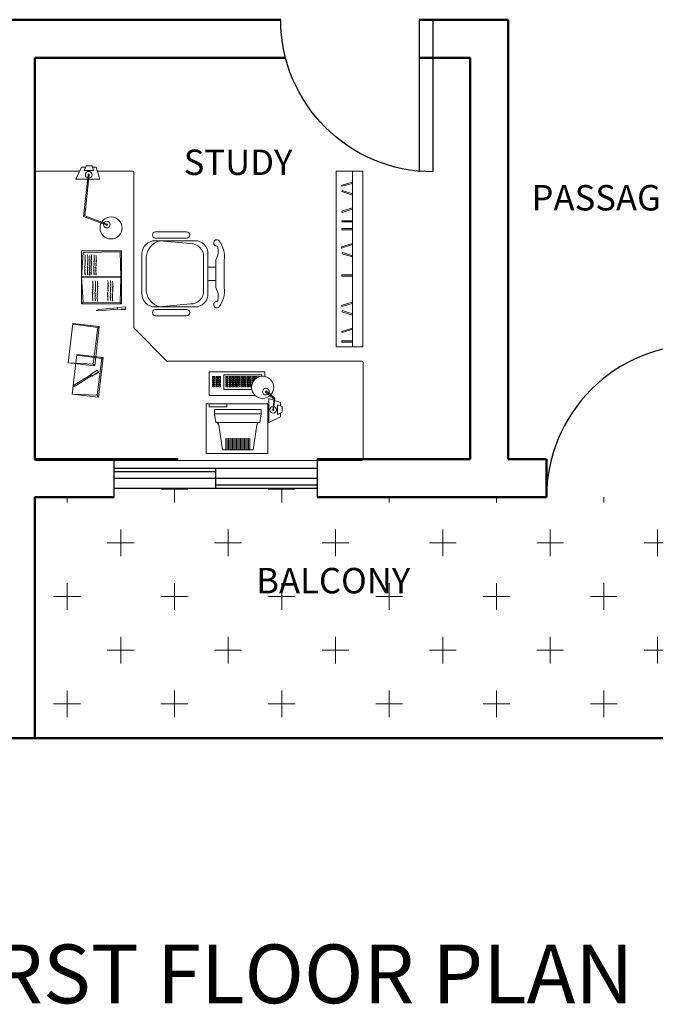
# Model space of a CAD drawing. Units: millimetres. Extents: x -857 to 54106, y -13666 to 13947.
# Tile 17 of 41: x 24780 to 28540, y 2329 to 8154. Entities that reach past the tile are written whole.
import ezdxf

# ---------------------------------------------------------------- set-up
doc = ezdxf.new("R2010")
doc.units = ezdxf.units.MM
for name, color, linetype, lineweight in [('A-ANNO-TEXT', 7, 'Continuous', 25), ('A-AREA-IDEN', 3, 'Continuous', 18), ('A-DOOR', 1, 'Continuous', 25), ('A-FLOR-PATT', 252, 'Continuous', 13), ('A-FURN', 21, 'Continuous', 18), ('A-GLAZ', 4, 'Continuous', 25), ('A-WALL', 7, 'Continuous', 50)]:
    doc.layers.add(name, color=color, linetype=linetype, lineweight=lineweight)
doc.styles.get("Standard").update_dxf_attribs({"font": 'arial.ttf'})

# ---------------------------------------------------------------- blocks, each defined once
blk = doc.blocks.new('DOOR-900')
blk.add_line((11417.3, 9811.5), (12317.3, 9811.5))
blk.add_arc((11417.3, 9811.5), 900, 0, 90)
blk = doc.blocks.new('WIN-1200')
for p, q in [((9371.3, 11750.2), (10571.3, 11750.2)), ((9371.3, 11731.7), (9971.3, 11731.7)), ((9971.3, 11750.2), (9971.3, 11630.7)), ((9371.3, 11691.7), (10571.3, 11691.7)), ((9971.3, 11651.7), (10571.3, 11651.7)), ((10571.3, 11630.7), (9371.3, 11630.7))]:
    blk.add_line(p, q)
for points in [[(9371.3, 11579.2), (9371.3, 11804.2)], [(10571.3, 11804.2), (10571.3, 11579.2)]]:
    blk.add_lwpolyline(points)

msp = doc.modelspace()

# ---------------------------------------------------------------- hatches: boundary and pattern name
at = {"layer": 'A-FLOR-PATT'}
h = msp.add_hatch(dxfattribs=at)
h.set_pattern_fill('CROSS', color=256, scale=50)
h.set_pattern_definition([(0, (11962.88, -2561.3), (317.5, 317.5), [158.75, -476.25]), (90, (12042.26, -2640.7), (-317.5, 317.5), [158.75, -476.25])])
h.paths.add_polyline_path([(29079.919, 5329.231), (28716.385, 5329.231), (27076.385, 5329.231), (26996.385, 5329.231), (26539.053, 5329.231), (26539.053, 5380.706), (25339.053, 5380.706), (25339.053, 5329.231), (24870.079, 5329.231), (24870.079, 3903.799), (29079.919, 3903.799)])

# ---------------------------------------------------------------- linework, layer by layer
at = {"layer": 'A-DOOR'}
msp.add_line((27143.761, 8154.231), (27143.761, 7254.231), dxfattribs=at)
at = {"layer": 'A-FURN'}
for p, q in [((25160.508, 7261.556), (25173.98, 7289.341)), ((25208.191, 7289.341), (25173.98, 7289.341)), ((25208.191, 7289.341), (25217.357, 7261.556)), ((25112.268, 7211.399), (25145.95, 7280.862)), ((25169.869, 7280.862), (25145.95, 7280.862)), ((25184.32, 7235.602), (25158.173, 6990.396)), ((25217.357, 7261.556), (25160.508, 7261.556)), ((25191.68, 7238.315), (25165.182, 6994.061)), ((25231.476, 7280.862), (25210.988, 7280.862)), ((25231.476, 7280.862), (25254.392, 7211.399)), ((26652.793, 7258.702), (26652.793, 6219.198)), ((26652.793, 7258.702), (26810.205, 7258.702)), ((26748.886, 7258.702), (26748.886, 6219.198)), ((26810.205, 6219.198), (26810.205, 7258.702)), ((25254.392, 7211.399), (25112.268, 7211.399)), ((25158.173, 6990.396), (25291.756, 6940.082)), ((25165.182, 6994.061), (25298.184, 6944.578)), ((25581.356, 6899.415), (25767.4, 6899.415)), ((25581.356, 6861.617), (25767.4, 6861.617)), ((25155.775, 6777.447), (25146.069, 6630.683)), ((25375.038, 6780.342), (25155.775, 6777.447)), ((25375.038, 6780.342), (25378.51, 6633.881)), ((25893.633, 6690.024), (25939.644, 6690.024)), ((25378.51, 6633.881), (25146.069, 6633.881)), ((25155.775, 6483.92), (25146.069, 6630.683)), ((25375.038, 6481.025), (25378.51, 6627.485)), ((25378.51, 6627.485), (25381.257, 6630.659)), ((25893.633, 6611.58), (25939.644, 6611.58)), ((25146.069, 6473.796), (25155.775, 6483.92)), ((25375.038, 6481.025), (25155.775, 6483.92)), ((25381.399, 6473.796), (25375.038, 6481.025)), ((25246.61, 6439.514), (25232.761, 6433.905)), ((25232.761, 6433.905), (25247.32, 6431.702)), ((25358.654, 6449.693), (25246.61, 6439.514)), ((25359.364, 6441.881), (25247.32, 6431.702)), ((25358.465, 6451.781), (25405.161, 6456.024)), ((25358.654, 6449.693), (25358.465, 6451.781)), ((25359.544, 6438.967), (25358.57, 6449.686)), ((25406.325, 6443.217), (25359.544, 6438.967)), ((25404.946, 6443.883), (25382.156, 6441.813)), ((25382.156, 6441.813), (25382.459, 6438.476)), ((25405.249, 6440.546), (25382.459, 6438.476)), ((25404.946, 6443.883), (25405.249, 6440.546)), ((25405.161, 6456.024), (25406.325, 6443.217)), ((25581.356, 6439.986), (25767.4, 6439.986)), ((25096.866, 6353.896), (25094.021, 6356.983)), ((25242.011, 6334.005), (25096.866, 6353.896)), ((25581.356, 6402.189), (25767.4, 6402.189)), ((25242.011, 6334.005), (25214.52, 6116.453)), ((25249.908, 6339.515), (25242.011, 6334.005)), ((25650.994, 6134.713), (25454.885, 6330.671)), ((26652.793, 6219.198), (26810.205, 6219.198)), ((25214.52, 6116.453), (25067.595, 6123.284)), ((25120.179, 6170.198), (25117.333, 6173.285)), ((25265.323, 6150.308), (25120.179, 6170.198)), ((25223.49, 6105.672), (25214.52, 6116.453)), ((25265.323, 6150.308), (25237.833, 5932.755)), ((25265.323, 6150.308), (25273.22, 6155.817)), ((25199.076, 6055.795), (25238.723, 6080.829)), ((25245.589, 6069.956), (25205.871, 6044.876)), ((25244.058, 6069.921), (25224.709, 6057.704)), ((25245.846, 6067.088), (25226.498, 6054.871)), ((25238.723, 6080.829), (25245.589, 6069.956)), ((25244.058, 6069.921), (25245.846, 6067.088)), ((26229.928, 6070.027), (25901.209, 6070.027)), ((25901.209, 6070.027), (25901.209, 5931.619)), ((26229.928, 6043.131), (26229.928, 6070.027)), ((25200.196, 6054.022), (25105.067, 5993.955)), ((25204.384, 6047.389), (25109.255, 5987.322)), ((25200.196, 6054.022), (25199.076, 6055.795)), ((25205.871, 6044.876), (25200.124, 6053.977)), ((25224.709, 6057.704), (25226.498, 6054.871)), ((26212.627, 6052.726), (25987.714, 6052.726)), ((25987.714, 6052.726), (25987.714, 5966.221)), ((26212.627, 6044.227), (26212.627, 6052.726)), ((25105.067, 5993.955), (25095.29, 5982.656)), ((25095.29, 5982.656), (25109.255, 5987.322)), ((25987.714, 5966.221), (26152.903, 5966.221)), ((26285.149, 5908.373), (26234.835, 5949.996)), ((26288.815, 5915.382), (26239.332, 5956.423)), ((25237.833, 5932.755), (25090.907, 5939.586)), ((25246.802, 5921.974), (25237.833, 5932.755)), ((25901.209, 5931.619), (26171.815, 5931.619)), ((26253.814, 5912.631), (26253.814, 5770.508)), ((26323.277, 5889.716), (26253.814, 5912.631)), ((26278.016, 5842.559), (26285.149, 5908.373)), ((26280.73, 5849.919), (26288.815, 5915.382)), ((26323.277, 5889.716), (26323.277, 5869.227)), ((26247.151, 5881.979), (25883.829, 5881.979)), ((25883.829, 5881.979), (25883.829, 5587.862)), ((25901.13, 5881.979), (25901.13, 5864.678)), ((25901.13, 5864.678), (26004.936, 5864.678)), ((26207.734, 5847.871), (25931.613, 5847.871)), ((25931.613, 5847.871), (25931.613, 5823.408)), ((26004.936, 5864.678), (26004.936, 5881.979)), ((26207.734, 5823.408), (26207.734, 5847.871)), ((26247.151, 5587.862), (26247.151, 5881.979)), ((26303.97, 5875.597), (26303.97, 5818.747)), ((26331.756, 5866.43), (26303.97, 5875.597)), ((26303.97, 5818.747), (26331.756, 5832.22)), ((26323.277, 5828.109), (26323.277, 5804.189)), ((26331.756, 5866.43), (26331.756, 5832.22)), ((25931.613, 5823.408), (26207.734, 5823.408)), ((25931.613, 5823.408), (25939.595, 5770.488)), ((26199.982, 5770.488), (25939.595, 5770.488)), ((26199.982, 5770.488), (26207.734, 5823.408)), ((26253.814, 5770.508), (26323.277, 5804.189)), ((25978.907, 5610.358), (25957.543, 5756.207)), ((26160.67, 5610.358), (26182.034, 5756.207)), ((25999.538, 5610.358), (25999.538, 5679.223)), ((26007.383, 5610.358), (26007.383, 5679.223)), ((26015.227, 5610.358), (26015.227, 5679.223)), ((26023.071, 5610.358), (26023.071, 5679.223)), ((26030.916, 5610.358), (26030.916, 5679.223)), ((26038.76, 5610.358), (26038.76, 5679.223)), ((26046.604, 5610.358), (26046.604, 5679.223)), ((26054.449, 5610.358), (26054.449, 5679.223)), ((26054.449, 5610.358), (26054.449, 5679.223)), ((26062.293, 5610.358), (26062.293, 5679.223)), ((26070.137, 5610.358), (26070.137, 5679.223)), ((26077.982, 5610.358), (26077.982, 5679.223)), ((26085.826, 5610.358), (26085.826, 5679.223)), ((26093.67, 5610.358), (26093.67, 5679.223)), ((26101.515, 5610.358), (26101.515, 5679.223)), ((26109.359, 5610.358), (26109.359, 5679.223)), ((26117.204, 5610.358), (26117.204, 5679.223)), ((26125.048, 5610.358), (26125.048, 5679.223)), ((26132.892, 5610.358), (26132.892, 5679.223)), ((26140.737, 5610.358), (26140.737, 5679.223)), ((25978.907, 5610.358), (26160.67, 5610.358)), ((25883.829, 5587.862), (26247.151, 5587.862))]:
    msp.add_line(p, q, dxfattribs=at)
for points in [[(25447.04, 5546.387), (24874.403, 5546.387, -0.41421356), (24866.558, 5554.231), (24866.558, 7250.857, -0.41421356), (24874.403, 7258.702), (25135.205, 7258.702)], [(25238.787, 7258.702), (25447.04, 7258.702, -0.41421356), (25454.885, 7250.857), (25454.885, 6330.671)], [(25502.985, 6650.802), (25502.985, 6768.467, -0.41421356), (25581.428, 6846.911), (25816.759, 6846.911, -0.41837619), (25893.633, 6768.467), (25893.633, 6650.802)], [(25527.65, 6650.802), (25527.65, 6750.867, -0.28027969), (25606.094, 6846.911), (25791.171, 6829.311, -0.41837619), (25868.045, 6750.867), (25868.045, 6650.802)], [(25956.196, 6850.36, -0.20706567), (25990.378, 6731.064), (25990.378, 6650.802)], [(25949.073, 6814.782, -0.21457838), (25939.644, 6731.387), (25939.644, 6650.802)], [(25502.985, 6650.802), (25502.985, 6533.137, 0.41421356), (25581.428, 6454.693), (25816.759, 6454.693, 0.41837619), (25893.633, 6533.137), (25893.633, 6650.802)], [(25527.65, 6650.802), (25527.65, 6550.736, 0.28027969), (25606.094, 6454.693), (25791.171, 6472.293, 0.41837619), (25868.045, 6550.736), (25868.045, 6650.802)], [(25949.073, 6486.822, 0.21457838), (25939.644, 6570.217), (25939.644, 6650.802)], [(25956.196, 6451.244, 0.20706567), (25990.378, 6570.54), (25990.378, 6650.802)], [(25650.994, 6134.713), (26804.658, 6134.713, -0.41421356), (26812.503, 6126.869), (26812.503, 5554.231, -0.41421356), (26804.658, 5546.387), (25447.04, 5546.387)]]:
    msp.add_lwpolyline(points, format="xyb", dxfattribs=at)
for points in [[(26748.886, 7185.97), (26686.412, 7169.063), (26685.22, 7175.896), (26748.886, 7193.127)], [(26748.886, 7116.919), (26686.222, 7136.927), (26687.616, 7143.722), (26748.886, 7124.159)], [(26748.886, 7040.642), (26686.222, 7020.633), (26687.616, 7013.838), (26748.886, 7033.401)], [(26748.886, 6958.009), (26685.22, 6958.009), (26685.22, 6964.946), (26748.886, 6964.946)], [(26748.886, 6911.186), (26685.22, 6911.186), (26685.22, 6918.122), (26748.886, 6918.122)], [(26748.886, 6830.798), (26682.756, 6809.683), (26684.15, 6802.888), (26748.886, 6823.558)], [(26748.886, 6750.443), (26687.955, 6769.898), (26689.349, 6776.693), (26748.886, 6757.683)], [(26748.886, 6637.18), (26685.22, 6637.18), (26685.22, 6644.116), (26748.886, 6644.116)], [(26748.886, 6475.333), (26686.412, 6458.425), (26685.22, 6465.259), (26748.886, 6482.489)], [(26748.886, 6406.281), (26686.222, 6426.29), (26687.616, 6433.085), (26748.886, 6413.522)], [(26748.886, 6330.004), (26686.222, 6309.996), (26687.616, 6303.201), (26748.886, 6322.764)], [(26748.886, 6247.372), (26685.22, 6247.372), (26685.22, 6254.309), (26748.886, 6254.309)], [(26162.58, 6015.079), (26157.798, 6015.079), (26157.798, 6021.383), (26167.33, 6021.383)], [(26157.798, 6006.546), (26157.798, 6011.2), (26160.197, 6011.2)], [(26174.295, 6028.401), (26174.295, 6032.536), (26179.599, 6032.536)], [(26193.219, 6039.847), (26193.219, 6043.204), (26204.379, 6043.204), (26204.379, 6043.123)]]:
    msp.add_lwpolyline(points, dxfattribs=at)
for points in [[(25381.399, 6630.683), (25381.399, 6787.57), (25146.069, 6787.57), (25146.069, 6630.683)], [(25381.399, 6630.683), (25381.399, 6473.796), (25146.069, 6473.796), (25146.069, 6630.683)], [(25094.013, 6357.127), (25249.908, 6339.515), (25223.49, 6105.672), (25067.595, 6123.284)], [(25117.325, 6173.429), (25273.22, 6155.817), (25246.802, 5921.974), (25090.907, 5939.586)], [(25920.524, 6043.204), (25931.684, 6043.204), (25931.684, 6036.9), (25920.524, 6036.9)], [(25920.524, 6032.536), (25931.684, 6032.536), (25931.684, 6026.232), (25920.524, 6026.232)], [(25920.524, 6021.383), (25931.684, 6021.383), (25931.684, 6015.079), (25920.524, 6015.079)], [(25920.524, 6011.2), (25931.684, 6011.2), (25931.684, 6004.896), (25920.524, 6004.896)], [(25920.524, 6000.532), (25931.684, 6000.532), (25931.684, 5994.228), (25920.524, 5994.228)], [(25939.448, 6043.204), (25950.608, 6043.204), (25950.608, 6036.9), (25939.448, 6036.9)], [(25939.448, 6032.536), (25950.608, 6032.536), (25950.608, 6026.232), (25939.448, 6026.232)], [(25939.448, 6021.383), (25950.608, 6021.383), (25950.608, 6015.079), (25939.448, 6015.079)], [(25939.448, 6011.2), (25950.608, 6011.2), (25950.608, 6004.896), (25939.448, 6004.896)], [(25939.448, 6000.532), (25950.608, 6000.532), (25950.608, 5994.228), (25939.448, 5994.228)], [(25955.945, 6043.204), (25967.106, 6043.204), (25967.106, 6036.9), (25955.945, 6036.9)], [(25955.945, 6032.536), (25967.106, 6032.536), (25967.106, 6026.232), (25955.945, 6026.232)], [(25955.945, 6021.383), (25967.106, 6021.383), (25967.106, 6015.079), (25955.945, 6015.079)], [(25955.945, 6011.2), (25967.106, 6011.2), (25967.106, 6004.896), (25955.945, 6004.896)], [(25955.945, 6000.532), (25967.106, 6000.532), (25967.106, 5994.228), (25955.945, 5994.228)], [(25999.13, 6043.204), (26010.29, 6043.204), (26010.29, 6036.9), (25999.13, 6036.9)], [(25999.13, 6032.536), (26010.29, 6032.536), (26010.29, 6026.232), (25999.13, 6026.232)], [(25999.13, 6021.383), (26010.29, 6021.383), (26010.29, 6015.079), (25999.13, 6015.079)], [(25999.13, 6011.2), (26010.29, 6011.2), (26010.29, 6004.896), (25999.13, 6004.896)], [(25999.13, 6000.532), (26010.29, 6000.532), (26010.29, 5994.228), (25999.13, 5994.228)], [(26018.054, 6043.204), (26029.214, 6043.204), (26029.214, 6036.9), (26018.054, 6036.9)], [(26018.054, 6032.536), (26029.214, 6032.536), (26029.214, 6026.232), (26018.054, 6026.232)], [(26018.054, 6021.383), (26029.214, 6021.383), (26029.214, 6015.079), (26018.054, 6015.079)], [(26018.054, 6011.2), (26029.214, 6011.2), (26029.214, 6004.896), (26018.054, 6004.896)], [(26018.054, 6000.532), (26029.214, 6000.532), (26029.214, 5994.228), (26018.054, 5994.228)], [(26034.551, 6043.204), (26045.712, 6043.204), (26045.712, 6036.9), (26034.551, 6036.9)], [(26034.551, 6032.536), (26045.712, 6032.536), (26045.712, 6026.232), (26034.551, 6026.232)], [(26034.551, 6021.383), (26045.712, 6021.383), (26045.712, 6015.079), (26034.551, 6015.079)], [(26034.551, 6011.2), (26045.712, 6011.2), (26045.712, 6004.896), (26034.551, 6004.896)], [(26034.551, 6000.532), (26045.712, 6000.532), (26045.712, 5994.228), (26034.551, 5994.228)], [(26053.475, 6043.204), (26064.635, 6043.204), (26064.635, 6036.9), (26053.475, 6036.9)], [(26053.475, 6032.536), (26064.635, 6032.536), (26064.635, 6026.232), (26053.475, 6026.232)], [(26053.475, 6021.383), (26064.635, 6021.383), (26064.635, 6015.079), (26053.475, 6015.079)], [(26053.475, 6011.2), (26064.635, 6011.2), (26064.635, 6004.896), (26053.475, 6004.896)], [(26053.475, 6000.532), (26064.635, 6000.532), (26064.635, 5994.228), (26053.475, 5994.228)], [(26068.517, 6043.204), (26079.677, 6043.204), (26079.677, 6036.9), (26068.517, 6036.9)], [(26068.517, 6032.536), (26079.677, 6032.536), (26079.677, 6026.232), (26068.517, 6026.232)], [(26068.517, 6021.383), (26079.677, 6021.383), (26079.677, 6015.079), (26068.517, 6015.079)], [(26068.517, 6011.2), (26079.677, 6011.2), (26079.677, 6004.896), (26068.517, 6004.896)], [(26068.517, 6000.532), (26079.677, 6000.532), (26079.677, 5994.228), (26068.517, 5994.228)], [(26087.441, 6043.204), (26098.601, 6043.204), (26098.601, 6036.9), (26087.441, 6036.9)], [(26087.441, 6032.536), (26098.601, 6032.536), (26098.601, 6026.232), (26087.441, 6026.232)], [(26087.441, 6021.383), (26098.601, 6021.383), (26098.601, 6015.079), (26087.441, 6015.079)], [(26087.441, 6011.2), (26098.601, 6011.2), (26098.601, 6004.896), (26087.441, 6004.896)], [(26087.441, 6000.532), (26098.601, 6000.532), (26098.601, 5994.228), (26087.441, 5994.228)], [(26103.938, 6043.204), (26115.098, 6043.204), (26115.098, 6036.9), (26103.938, 6036.9)], [(26103.938, 6032.536), (26115.098, 6032.536), (26115.098, 6026.232), (26103.938, 6026.232)], [(26103.938, 6021.383), (26115.098, 6021.383), (26115.098, 6015.079), (26103.938, 6015.079)], [(26103.938, 6011.2), (26115.098, 6011.2), (26115.098, 6004.896), (26103.938, 6004.896)], [(26103.938, 6000.532), (26115.098, 6000.532), (26115.098, 5994.228), (26103.938, 5994.228)], [(26122.862, 6043.204), (26134.022, 6043.204), (26134.022, 6036.9), (26122.862, 6036.9)], [(26122.862, 6032.536), (26134.022, 6032.536), (26134.022, 6026.232), (26122.862, 6026.232)], [(26122.862, 6021.383), (26134.022, 6021.383), (26134.022, 6015.079), (26122.862, 6015.079)], [(26122.862, 6011.2), (26134.022, 6011.2), (26134.022, 6004.896), (26122.862, 6004.896)], [(26122.862, 6000.532), (26134.022, 6000.532), (26134.022, 5994.228), (26122.862, 5994.228)], [(26138.874, 6043.204), (26150.034, 6043.204), (26150.034, 6036.9), (26138.874, 6036.9)], [(26138.874, 6032.536), (26150.034, 6032.536), (26150.034, 6026.232), (26138.874, 6026.232)], [(26138.874, 6021.383), (26150.034, 6021.383), (26150.034, 6015.079), (26138.874, 6015.079)], [(26138.874, 6011.2), (26150.034, 6011.2), (26150.034, 6004.896), (26138.874, 6004.896)], [(26138.874, 6000.532), (26150.034, 6000.532), (26150.034, 5994.228), (26138.874, 5994.228)], [(26157.798, 6043.204), (26168.958, 6043.204), (26168.958, 6036.9), (26157.798, 6036.9)], [(26157.798, 6032.536), (26168.958, 6032.536), (26168.958, 6026.232), (26157.798, 6026.232)], [(26174.295, 6043.204), (26185.456, 6043.204), (26185.456, 6036.9), (26174.295, 6036.9)], [(25920.524, 5989.378), (25931.684, 5989.378), (25931.684, 5983.075), (25920.524, 5983.075)], [(25939.448, 5989.378), (25950.608, 5989.378), (25950.608, 5983.075), (25939.448, 5983.075)], [(25955.945, 5989.378), (25967.106, 5989.378), (25967.106, 5983.075), (25955.945, 5983.075)], [(25999.13, 5989.378), (26010.29, 5989.378), (26010.29, 5983.075), (25999.13, 5983.075)], [(26018.054, 5989.378), (26029.214, 5989.378), (26029.214, 5983.075), (26018.054, 5983.075)], [(26034.551, 5989.378), (26045.712, 5989.378), (26045.712, 5983.075), (26034.551, 5983.075)], [(26053.475, 5989.378), (26064.635, 5989.378), (26064.635, 5983.075), (26053.475, 5983.075)], [(26068.517, 5989.378), (26079.677, 5989.378), (26079.677, 5983.075), (26068.517, 5983.075)], [(26087.441, 5989.378), (26098.601, 5989.378), (26098.601, 5983.075), (26087.441, 5983.075)], [(26103.938, 5989.378), (26115.098, 5989.378), (26115.098, 5983.075), (26103.938, 5983.075)], [(26122.862, 5989.378), (26134.022, 5989.378), (26134.022, 5983.075), (26122.862, 5983.075)], [(26138.874, 5989.378), (26150.034, 5989.378), (26150.034, 5983.075), (26138.874, 5983.075)]]:
    msp.add_lwpolyline(points, close=True, dxfattribs=at)
for centre, radius in [((25188, 7236.958), 19.765), ((25320.64, 6922.42), 65.505), ((25295.415, 6941.836), 19.765), ((26217.174, 5978.879), 65.505), ((26236.589, 5953.655), 19.765), ((26279.373, 5846.239), 19.765)]:
    msp.add_circle(centre, radius, dxfattribs=at)
for centre, radius, start, end in [((25188, 7236.958), 3.922, 20.2361973, 200.2361973), ((25294.97, 6942.33), 3.922, 214.9751188, 34.9751188), ((25584.878, 6880.553), 19.188, 100.5780631, 259.6419622), ((25767.4, 6880.516), 18.899, 270, 90), ((25946.559, 6833.787), 19.171, 59.8227994, 277.5348476), ((25946.559, 6467.816), 19.171, 82.4651524, 300.1772006), ((25584.806, 6421.111), 19.188, 100.3580378, 259.4219369), ((25767.4, 6421.088), 18.899, 270, 90), ((26237.084, 5953.21), 3.922, 55.0248818, 235.0248818), ((26279.373, 5846.239), 3.922, 249.7638026, 69.7638026), ((25940.429, 5753.117), 17.391, 6.4337599, 92.748041), ((26199.149, 5753.117), 17.391, 87.251959, 173.5662401)]:
    msp.add_arc(centre, radius, start, end, dxfattribs=at)
for points, knots in [([(25166.002, 6763.919), (25166.1, 6761.217), (25166.249, 6757.132), (25168.922, 6751.212), (25165.701, 6746.354), (25169.301, 6741.183), (25164.975, 6736.024), (25171.515, 6731.19), (25163.409, 6726.321), (25170.909, 6721.738), (25162.902, 6715.554), (25170.101, 6711.401), (25164.425, 6707.409), (25170.713, 6701.498), (25159.5, 6692.589), (25168.416, 6688.532), (25160.427, 6682.306), (25170.611, 6674.601), (25162.152, 6670.429), (25167.328, 6668.853), (25163.853, 6665.839), (25167.466, 6662.327), (25164.539, 6657.424), (25167.95, 6652.923), (25164.207, 6649.512), (25168.969, 6647.878), (25166.532, 6646.799), (25166.712, 6645.942), (25166.786, 6645.586)], [0, 0, 0, 0, 8.09206005, 12.23031262, 18.53000553, 22.52982456, 28.82951748, 33.21826518, 40.16259797, 43.70689848, 52.18430489, 55.72881041, 61.34252791, 63.49125817, 77.80948149, 80.61654327, 85.31692259, 97.40286307, 100.24093034, 103.04787013, 106.22169901, 108.46561095, 115.62707896, 119.59770326, 122.771583, 125.60958271, 127.02858257, 128.03248279, 128.03248279, 128.03248279, 128.03248279]), ([(25181.485, 6763.104), (25181.584, 6760.401), (25181.733, 6756.317), (25184.406, 6750.396), (25181.185, 6745.538), (25184.785, 6740.367), (25180.459, 6735.208), (25186.999, 6730.375), (25178.893, 6725.506), (25186.393, 6720.923), (25178.386, 6714.739), (25185.585, 6710.585), (25179.909, 6706.593), (25186.196, 6700.682), (25174.984, 6691.773), (25183.9, 6687.716), (25175.911, 6681.49), (25186.095, 6673.786), (25177.636, 6669.613), (25182.812, 6668.038), (25179.337, 6665.023), (25182.95, 6661.511), (25180.023, 6656.608), (25183.433, 6652.107), (25179.691, 6648.696), (25184.453, 6647.062), (25182.015, 6645.984), (25182.195, 6645.126), (25182.27, 6644.771)], [0, 0, 0, 0, 8.09206005, 12.23031263, 18.53000554, 22.52982457, 28.82951748, 33.21826519, 40.16259799, 43.70689848, 52.1843049, 55.72881042, 61.34252793, 63.49125817, 77.80948151, 80.61654329, 85.3169226, 97.40286307, 100.24093034, 103.04787013, 106.22169901, 108.46561095, 115.62707895, 119.59770325, 122.77158299, 125.6095827, 127.02858256, 128.03248278, 128.03248278, 128.03248278, 128.03248278]), ([(25193.709, 6759.842), (25193.808, 6757.139), (25193.957, 6753.055), (25196.63, 6747.134), (25193.409, 6742.276), (25197.009, 6737.106), (25192.683, 6731.947), (25199.223, 6727.113), (25191.117, 6722.244), (25198.617, 6717.661), (25190.61, 6711.477), (25197.809, 6707.323), (25192.133, 6703.331), (25198.42, 6697.421), (25187.208, 6688.512), (25196.124, 6684.455), (25188.135, 6678.228), (25198.319, 6670.524), (25189.86, 6666.352), (25195.036, 6664.776), (25191.561, 6661.761), (25195.174, 6658.25), (25192.247, 6653.346), (25195.657, 6648.845), (25191.915, 6645.435), (25196.677, 6643.801), (25194.239, 6642.722), (25194.419, 6641.864), (25194.494, 6641.509)], [0, 0, 0, 0, 8.09206003, 12.23031261, 18.53000552, 22.52982456, 28.82951746, 33.21826517, 40.16259797, 43.70689846, 52.18430488, 55.72881041, 61.34252791, 63.49125816, 77.8094815, 80.61654327, 85.31692259, 97.40286306, 100.24093034, 103.04787012, 106.22169899, 108.46561094, 115.62707894, 119.59770323, 122.77158297, 125.60958269, 127.02858255, 128.03248277, 128.03248277, 128.03248277, 128.03248277]), ([(25203.489, 6764.734), (25203.587, 6762.032), (25203.736, 6757.948), (25206.409, 6752.027), (25203.188, 6747.169), (25206.788, 6741.998), (25202.462, 6736.839), (25209.002, 6732.006), (25200.896, 6727.137), (25208.396, 6722.554), (25200.389, 6716.37), (25207.588, 6712.216), (25201.912, 6708.224), (25208.2, 6702.313), (25196.987, 6693.404), (25205.903, 6689.347), (25197.914, 6683.121), (25208.098, 6675.417), (25199.639, 6671.244), (25204.815, 6669.669), (25201.34, 6666.654), (25204.953, 6663.142), (25202.026, 6658.239), (25205.437, 6653.738), (25201.694, 6650.327), (25206.456, 6648.693), (25204.019, 6647.614), (25204.199, 6646.757), (25204.273, 6646.402)], [0, 0, 0, 0, 8.09206003, 12.23031261, 18.53000552, 22.52982456, 28.82951748, 33.21826519, 40.162598, 43.70689851, 52.18430493, 55.72881048, 61.34252799, 63.49125825, 77.80948159, 80.61654334, 85.31692264, 97.40286312, 100.24093041, 103.0478702, 106.22169907, 108.46561102, 115.62707902, 119.59770331, 122.77158305, 125.60958276, 127.02858262, 128.03248285, 128.03248285, 128.03248285, 128.03248285]), ([(25218.972, 6763.919), (25219.071, 6761.217), (25219.22, 6757.132), (25221.893, 6751.212), (25218.672, 6746.354), (25222.272, 6741.183), (25217.946, 6736.024), (25224.486, 6731.19), (25216.38, 6726.321), (25223.88, 6721.738), (25215.873, 6715.554), (25223.072, 6711.401), (25217.396, 6707.409), (25223.683, 6701.498), (25212.471, 6692.589), (25221.387, 6688.532), (25213.398, 6682.306), (25223.582, 6674.601), (25215.123, 6670.429), (25220.299, 6668.853), (25216.824, 6665.839), (25220.437, 6662.327), (25217.51, 6657.424), (25220.92, 6652.923), (25217.178, 6649.512), (25221.94, 6647.878), (25219.502, 6646.799), (25219.682, 6645.942), (25219.757, 6645.586)], [0, 0, 0, 0, 8.09206005, 12.23031262, 18.53000553, 22.52982456, 28.82951747, 33.21826518, 40.16259797, 43.70689848, 52.18430489, 55.72881041, 61.34252791, 63.49125817, 77.80948149, 80.61654327, 85.31692259, 97.40286306, 100.24093033, 103.04787012, 106.221699, 108.46561095, 115.62707896, 119.59770325, 122.77158299, 125.6095827, 127.02858256, 128.03248278, 128.03248278, 128.03248278, 128.03248278]), ([(25231.196, 6760.657), (25231.295, 6757.955), (25231.444, 6753.871), (25234.117, 6747.95), (25230.896, 6743.092), (25234.496, 6737.921), (25230.17, 6732.762), (25236.71, 6727.929), (25228.604, 6723.059), (25236.104, 6718.476), (25228.097, 6712.293), (25235.296, 6708.139), (25229.62, 6704.147), (25235.907, 6698.236), (25224.695, 6689.327), (25233.611, 6685.27), (25225.622, 6679.044), (25235.806, 6671.339), (25227.347, 6667.167), (25232.523, 6665.592), (25229.048, 6662.577), (25232.661, 6659.065), (25229.734, 6654.162), (25233.144, 6649.661), (25229.402, 6646.25), (25234.164, 6644.616), (25231.726, 6643.537), (25231.906, 6642.68), (25231.981, 6642.325)], [0, 0, 0, 0, 8.09206005, 12.23031263, 18.53000554, 22.52982458, 28.82951749, 33.21826521, 40.16259802, 43.70689853, 52.18430495, 55.7288105, 61.342528, 63.49125825, 77.80948159, 80.61654335, 85.31692266, 97.40286313, 100.2409304, 103.04787017, 106.22169905, 108.46561099, 115.62707899, 119.59770329, 122.77158303, 125.60958274, 127.0285826, 128.03248283, 128.03248283, 128.03248283, 128.03248283]), ([(25211.638, 6609.8), (25211.737, 6607.097), (25211.886, 6603.013), (25214.559, 6597.092), (25211.337, 6592.234), (25214.937, 6587.063), (25210.612, 6581.905), (25217.151, 6577.071), (25209.046, 6572.202), (25216.545, 6567.619), (25208.539, 6561.435), (25215.737, 6557.281), (25210.062, 6553.289), (25216.349, 6547.378), (25205.137, 6538.469), (25214.053, 6534.412), (25206.064, 6528.186), (25216.247, 6520.482), (25207.788, 6516.309), (25212.964, 6514.734), (25209.49, 6511.719), (25213.103, 6508.207), (25210.175, 6503.304), (25213.586, 6498.803), (25209.843, 6495.392), (25214.605, 6493.758), (25212.168, 6492.68), (25212.348, 6491.822), (25212.422, 6491.467)], [0, 0, 0, 0, 8.09206004, 12.23031261, 18.53000552, 22.52982457, 28.82951749, 33.21826519, 40.162598, 43.70689852, 52.18430494, 55.72881048, 61.34252799, 63.49125824, 77.80948158, 80.61654334, 85.31692265, 97.40286313, 100.24093042, 103.0478702, 106.22169907, 108.46561102, 115.62707902, 119.5977033, 122.77158304, 125.60958276, 127.02858262, 128.03248285, 128.03248285, 128.03248285, 128.03248285]), ([(25227.122, 6608.984), (25227.22, 6606.282), (25227.369, 6602.198), (25230.042, 6596.277), (25226.821, 6591.419), (25230.421, 6586.248), (25226.095, 6581.089), (25232.635, 6576.256), (25224.529, 6571.386), (25232.029, 6566.803), (25224.022, 6560.62), (25231.221, 6556.466), (25225.545, 6552.474), (25231.833, 6546.563), (25220.62, 6537.654), (25229.536, 6533.597), (25221.547, 6527.371), (25231.731, 6519.666), (25223.272, 6515.494), (25228.448, 6513.919), (25224.973, 6510.904), (25228.586, 6507.392), (25225.659, 6502.489), (25229.07, 6497.988), (25225.327, 6494.577), (25230.089, 6492.943), (25227.652, 6491.864), (25227.832, 6491.007), (25227.906, 6490.651)], [0, 0, 0, 0, 8.09206005, 12.23031262, 18.53000553, 22.52982456, 28.82951748, 33.21826518, 40.16259798, 43.70689848, 52.1843049, 55.72881042, 61.34252792, 63.49125817, 77.8094815, 80.61654328, 85.31692259, 97.40286306, 100.24093034, 103.04787012, 106.22169901, 108.46561095, 115.62707896, 119.59770326, 122.771583, 125.60958271, 127.02858257, 128.0324828, 128.0324828, 128.0324828, 128.0324828]), ([(25239.346, 6605.722), (25239.444, 6603.02), (25239.593, 6598.936), (25242.266, 6593.015), (25239.045, 6588.157), (25242.645, 6582.986), (25238.319, 6577.827), (25244.859, 6572.994), (25236.753, 6568.124), (25244.253, 6563.541), (25236.246, 6557.358), (25243.445, 6553.204), (25237.769, 6549.212), (25244.057, 6543.301), (25232.844, 6534.392), (25241.76, 6530.335), (25233.771, 6524.109), (25243.955, 6516.404), (25235.496, 6512.232), (25240.672, 6510.657), (25237.197, 6507.642), (25240.81, 6504.13), (25237.883, 6499.227), (25241.294, 6494.726), (25237.551, 6491.315), (25242.313, 6489.681), (25239.876, 6488.602), (25240.056, 6487.745), (25240.13, 6487.39)], [0, 0, 0, 0, 8.09206004, 12.23031262, 18.53000553, 22.52982457, 28.82951748, 33.2182652, 40.16259801, 43.70689852, 52.18430494, 55.72881048, 61.34252799, 63.49125824, 77.80948158, 80.61654334, 85.31692264, 97.40286311, 100.24093039, 103.04787016, 106.22169904, 108.46561097, 115.62707897, 119.59770327, 122.77158301, 125.60958273, 127.02858258, 128.03248282, 128.03248282, 128.03248282, 128.03248282]), ([(25301.281, 6611.43), (25301.379, 6608.728), (25301.528, 6604.644), (25304.201, 6598.723), (25300.98, 6593.865), (25304.58, 6588.694), (25300.254, 6583.535), (25306.794, 6578.702), (25298.688, 6573.833), (25306.188, 6569.25), (25298.181, 6563.066), (25305.38, 6558.912), (25299.705, 6554.92), (25305.992, 6549.009), (25294.78, 6540.1), (25303.695, 6536.043), (25295.707, 6529.817), (25305.89, 6522.113), (25297.431, 6517.94), (25302.607, 6516.365), (25299.133, 6513.35), (25302.745, 6509.838), (25299.818, 6504.935), (25303.229, 6500.434), (25299.486, 6497.023), (25304.248, 6495.389), (25301.811, 6494.311), (25301.991, 6493.453), (25302.065, 6493.098)], [0, 0, 0, 0, 8.09206005, 12.23031262, 18.53000553, 22.52982458, 28.82951749, 33.21826521, 40.16259802, 43.70689853, 52.18430495, 55.72881049, 61.34252801, 63.49125826, 77.80948159, 80.61654336, 85.31692266, 97.40286314, 100.24093041, 103.04787018, 106.22169905, 108.46561099, 115.627079, 119.59770329, 122.77158303, 125.60958274, 127.02858259, 128.03248282, 128.03248282, 128.03248282, 128.03248282]), ([(25316.764, 6610.615), (25316.863, 6607.913), (25317.012, 6603.829), (25319.685, 6597.908), (25316.464, 6593.05), (25320.064, 6587.879), (25315.738, 6582.72), (25322.278, 6577.886), (25314.172, 6573.017), (25321.672, 6568.434), (25313.665, 6562.25), (25320.864, 6558.097), (25315.188, 6554.105), (25321.476, 6548.194), (25310.263, 6539.285), (25319.179, 6535.228), (25311.19, 6529.002), (25321.374, 6521.297), (25312.915, 6517.125), (25318.091, 6515.549), (25314.616, 6512.535), (25318.229, 6509.023), (25315.302, 6504.12), (25318.712, 6499.619), (25314.97, 6496.208), (25319.732, 6494.574), (25317.295, 6493.495), (25317.474, 6492.638), (25317.549, 6492.282)], [0, 0, 0, 0, 8.09206004, 12.23031262, 18.53000553, 22.52982456, 28.82951746, 33.21826518, 40.16259798, 43.70689848, 52.18430489, 55.72881043, 61.34252792, 63.49125816, 77.8094815, 80.61654328, 85.31692259, 97.40286306, 100.24093034, 103.04787013, 106.22169901, 108.46561094, 115.62707894, 119.59770325, 122.77158299, 125.6095827, 127.02858255, 128.03248279, 128.03248279, 128.03248279, 128.03248279]), ([(25328.988, 6607.353), (25329.087, 6604.651), (25329.236, 6600.567), (25331.909, 6594.646), (25328.688, 6589.788), (25332.288, 6584.617), (25327.962, 6579.458), (25334.502, 6574.625), (25326.396, 6569.755), (25333.896, 6565.172), (25325.889, 6558.989), (25333.088, 6554.835), (25327.412, 6550.843), (25333.7, 6544.932), (25322.487, 6536.023), (25331.403, 6531.966), (25323.414, 6525.74), (25333.598, 6518.035), (25325.139, 6513.863), (25330.315, 6512.288), (25326.84, 6509.273), (25330.453, 6505.761), (25327.526, 6500.858), (25330.936, 6496.357), (25327.194, 6492.946), (25331.956, 6491.312), (25329.519, 6490.233), (25329.698, 6489.376), (25329.773, 6489.021)], [0, 0, 0, 0, 8.09206004, 12.23031261, 18.53000552, 22.52982456, 28.82951747, 33.21826517, 40.16259797, 43.70689847, 52.18430489, 55.72881041, 61.34252791, 63.49125816, 77.8094815, 80.61654327, 85.31692259, 97.40286307, 100.24093035, 103.04787012, 106.22169901, 108.46561096, 115.62707896, 119.59770326, 122.771583, 125.60958271, 127.02858257, 128.0324828, 128.0324828, 128.0324828, 128.0324828])]:
    msp.add_open_spline(points, degree=3, knots=knots, dxfattribs=at)
at = {"layer": 'A-WALL'}
for p, q in [((24645.079, 8154.231), (24870.079, 8154.231)), ((24870.079, 8154.231), (26323.761, 8154.231)), ((27143.761, 8154.231), (27670.079, 8154.231)), ((27670.079, 8154.231), (27670.079, 5554.231)), ((24870.079, 7929.231), (24870.079, 5554.231)), ((24870.079, 5554.231), (24870.079, 7929.231)), ((24870.079, 7929.231), (26352.339, 7929.231)), ((27143.761, 7929.231), (27445.079, 7929.231)), ((27445.079, 7929.231), (27445.079, 5554.231)), ((24866.558, 5554.231), (25717.422, 5554.231)), ((26539.053, 5554.231), (27076.385, 5554.231)), ((27076.385, 5554.231), (26922.69, 5554.231)), ((27445.079, 5554.231), (27076.385, 5554.231)), ((27670.079, 5554.231), (27896.385, 5554.231)), ((27896.385, 5329.231), (27896.385, 5554.231)), ((27076.385, 5329.231), (27896.385, 5329.231)), ((23593.518, 3904.023), (24870.079, 3904.023))]:
    msp.add_line(p, q, dxfattribs=at)
for points in [[(25339.053, 5329.231), (24870.079, 5329.231), (24870.079, 3903.799)], [(25339.053, 5329.231), (24870.079, 5329.231), (24870.079, 3903.799), (29079.919, 3903.799), (29079.919, 5329.231), (28716.385, 5329.231)], [(27076.385, 5329.231), (26539.053, 5329.231)], [(27076.385, 5329.231), (26539.053, 5329.231)]]:
    msp.add_lwpolyline(points, dxfattribs=at)

# ---------------------------------------------------------------- block references
at = {"layer": 'A-DOOR', "extrusion": (0, 0, -1), "zscale": -1, "rotation": 269.9999999999999}
msp.add_blockref('DOOR-900', (-37035.242, 19571.511), dxfattribs=at)
at = {"layer": 'A-DOOR', "rotation": 89.99999999999991}
msp.add_blockref('DOOR-900', (38607.866, -6088.049), dxfattribs=at)
at = {"layer": 'A-GLAZ'}
msp.add_blockref('WIN-1200', (15967.712, -6250), dxfattribs=at)

# ---------------------------------------------------------------- texts
at = {"layer": 'A-ANNO-TEXT', "insert": (24215.858, 2682.963), "char_height": 347.60543, "attachment_point": 1}
msp.add_mtext_dynamic_manual_height_columns('\\pxt0;FIRST FLOOR PLAN', width=5900.0263, gutter_width=43450.679, heights=[5996.136], dxfattribs=at)
at = {"layer": 'A-AREA-IDEN', "char_height": 150.48461, "attachment_point": 1}
for s, insert in [('\\pxt0;STUDY', (25749.879, 7385.961)), ('\\pxt0;PASSAGE', (27807.484, 7176.075)), ('\\pxt0;BALCONY', (26178.66, 4910.875))]:
    msp.add_mtext_dynamic_manual_height_columns(s, width=2554.22693, gutter_width=18810.576, heights=[2595.835], dxfattribs=dict(at, insert=insert))

doc.saveas('drawing.dxf')
